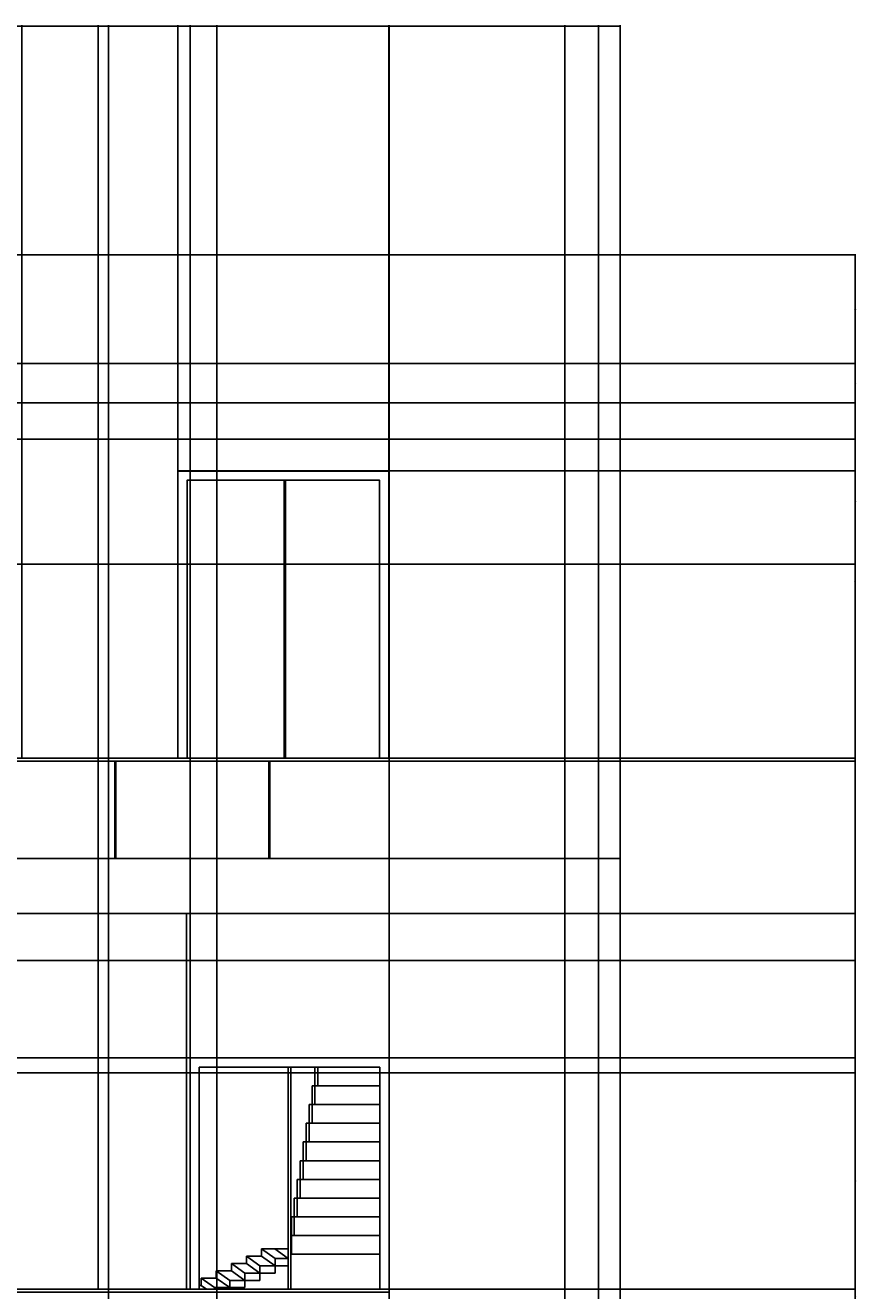
# Model space of a CAD drawing. Units: feet. Extents: x 2193 to 3502, y 890 to 1601.
# Tile 17 of 17: x 3283 to 3502, y 1268 to 1601. Entities that reach past the tile are written whole.
import ezdxf

# ---------------------------------------------------------------- set-up
doc = ezdxf.new("R2010")
doc.units = ezdxf.units.FT
doc.layers.add('A-ANNO-DIMS', color=2, linetype='Continuous', lineweight=18)
doc.layers.add('A-ELEV', color=7, linetype='Continuous', lineweight=25)
doc.styles.get("Standard").update_dxf_attribs({"font": 'arial.ttf'})
doc.dimstyles.get("Standard").update_dxf_attribs({"dimtxt": 0.18, "dimasz": 0.18, "dimexe": 0.18, "dimexo": 0.0625, "dimgap": 0.09, "dimtad": 0, "dimtih": 1, "dimtoh": 1, "dimdec": 0, "dimzin": 0, "dimdsep": 46, "dimlunit": 3, "dimtxsty": 'Standard', "dimcen": 0.09, "dimadec": 0, "dimazin": 0, "dimtfac": 1, "dimtdec": 0, "dimtofl": 0, "dimtmove": 0, "dimatfit": 3, "dimfxl": 1, "dimtolj": 1, "dimtzin": 0, "dimarcsym": 0})

# ---------------------------------------------------------------- blocks, each defined once
blk = doc.blocks.new('STAIR-RAIL-B')
for p, q in [((6.38, 44.29), (6.38, 49.22)), ((5.61, 39.37), (5.61, 44.29)), ((5.61, 44.29), (6.38, 44.29)), ((23.45, 44.29), (6.38, 44.29)), ((6.38, 44.29), (6.38, 39.37)), ((4.83, 34.45), (4.83, 39.37)), ((4.83, 39.37), (5.61, 39.37)), ((23.45, 39.37), (5.61, 39.37)), ((5.61, 39.37), (5.61, 34.45)), ((4.05, 29.53), (4.05, 34.45)), ((4.05, 34.45), (4.83, 34.45)), ((23.45, 34.45), (4.83, 34.45)), ((4.83, 34.45), (4.83, 29.53)), ((3.27, 24.61), (3.27, 29.53)), ((3.27, 29.53), (4.05, 29.53)), ((23.45, 29.53), (4.05, 29.53)), ((4.05, 29.53), (4.05, 24.61)), ((2.49, 19.69), (2.49, 24.61)), ((2.49, 24.61), (3.27, 24.61)), ((23.45, 24.61), (3.27, 24.61)), ((3.27, 24.61), (3.27, 19.69)), ((1.71, 14.77), (1.71, 19.69)), ((1.71, 19.69), (2.49, 19.69)), ((23.45, 19.69), (2.49, 19.69)), ((2.49, 19.69), (2.49, 14.77)), ((0.93, 9.84), (0.93, 14.77)), ((0.93, 14.77), (1.71, 14.77)), ((23.45, 14.77), (1.71, 14.77)), ((1.71, 14.77), (1.71, 9.84)), ((0.15, 4.92), (0.15, 9.84)), ((0.15, 9.84), (0.93, 9.84)), ((23.45, 9.84), (0.93, 9.84)), ((0.93, 9.84), (0.93, 4.92)), ((23.45, 4.92), (0, 4.92)), ((0.15, 4.92), (0.15, 0)), ((23.45, 0), (0, 0))]:
    blk.add_line(p, q)
blk = doc.blocks.new('*D13')
at = {"layer": 'A-ANNO-DIMS', "color": 0, "lineweight": -2, "transparency": 16777216}
for p, q in [((2934.37, 950.89), (2934.37, 1601.47)), ((2934.55, 1601.29), (3186.64, 1601.29)), ((3439.51, 1601.29), (3187.43, 1601.29)), ((3439.69, 1541.11), (3439.69, 1601.47))]:
    blk.add_line(p, q, dxfattribs=at)
at = {"layer": 'A-ANNO-DIMS', "color": 0, "transparency": 16777216}
for points in [[(2934.55, 1601.32), (2934.55, 1601.26), (2934.37, 1601.29)], [(3439.51, 1601.32), (3439.51, 1601.26), (3439.69, 1601.29)]]:
    blk.add_solid(points, dxfattribs=at)
at = {"layer": 'Defpoints', "color": 0, "transparency": 16777216}
for p in [(3439.69, 1601.29), (3439.69, 1541.04), (2934.37, 950.82)]:
    blk.add_point(p, dxfattribs=at)
at = {"layer": 'A-ANNO-DIMS', "color": 0, "transparency": 16777216, "insert": (3187.03, 1601.29), "char_height": 0.18, "attachment_point": 5}
blk.add_mtext('\\A1;505.3', dxfattribs=at)
blk = doc.blocks.new('*D18')
at = {"layer": 'A-ANNO-DIMS', "color": 0, "lineweight": -2, "transparency": 16777216}
for p, q in [((3439.75, 1541.04), (3501.85, 1541.04)), ((3501.67, 1540.86), (3501.67, 1246.12)), ((3501.67, 951), (3501.67, 1245.75)), ((3441.48, 950.82), (3501.85, 950.82))]:
    blk.add_line(p, q, dxfattribs=at)
at = {"layer": 'A-ANNO-DIMS', "color": 0, "transparency": 16777216}
for points in [[(3501.64, 1540.86), (3501.7, 1540.86), (3501.67, 1541.04)], [(3501.64, 951), (3501.7, 951), (3501.67, 950.82)]]:
    blk.add_solid(points, dxfattribs=at)
at = {"layer": 'Defpoints', "color": 0, "transparency": 16777216}
for p in [(3439.69, 1541.04), (3501.67, 1541.04), (3441.42, 950.82)]:
    blk.add_point(p, dxfattribs=at)
at = {"layer": 'A-ANNO-DIMS', "color": 0, "transparency": 16777216, "insert": (3501.67, 1245.93), "char_height": 0.18, "attachment_point": 5}
blk.add_mtext('\\A1;590.2', dxfattribs=at)
blk = doc.blocks.new('*D31')
at = {"layer": 'A-ANNO-DIMS', "color": 0, "lineweight": -2, "transparency": 16777216}
for p, q in [((2760.54, 1541.04), (3501.85, 1541.04)), ((3501.67, 1540.86), (3501.67, 1246.12)), ((3501.67, 951), (3501.67, 1245.75)), ((2762.27, 950.82), (3501.85, 950.82))]:
    blk.add_line(p, q, dxfattribs=at)
at = {"layer": 'A-ANNO-DIMS', "color": 0, "transparency": 16777216}
for points in [[(3501.64, 1540.86), (3501.7, 1540.86), (3501.67, 1541.04)], [(3501.64, 951), (3501.7, 951), (3501.67, 950.82)]]:
    blk.add_solid(points, dxfattribs=at)
at = {"layer": 'Defpoints', "color": 0, "transparency": 16777216}
for p in [(2760.47, 1541.04), (3501.67, 1541.04), (2762.2, 950.82)]:
    blk.add_point(p, dxfattribs=at)
at = {"layer": 'A-ANNO-DIMS', "color": 0, "transparency": 16777216, "insert": (3501.67, 1245.93), "char_height": 0.18, "attachment_point": 5}
blk.add_mtext('\\A1;590.2', dxfattribs=at)
blk = doc.blocks.new('*D40')
at = {"layer": 'A-ANNO-DIMS', "color": 0, "lineweight": -2, "transparency": 16777216}
for p, q in [((3378.91, 1502.08), (3501.85, 1502.08)), ((3501.67, 1501.9), (3501.67, 1455.09)), ((3501.67, 1407.92), (3501.67, 1454.73)), ((3378.85, 1407.74), (3501.85, 1407.74))]:
    blk.add_line(p, q, dxfattribs=at)
at = {"layer": 'A-ANNO-DIMS', "color": 0, "transparency": 16777216}
for points in [[(3501.64, 1501.9), (3501.7, 1501.9), (3501.67, 1502.08)], [(3501.64, 1407.92), (3501.7, 1407.92), (3501.67, 1407.74)]]:
    blk.add_solid(points, dxfattribs=at)
at = {"layer": 'Defpoints', "color": 0, "transparency": 16777216}
for p in [(3378.85, 1502.08), (3501.67, 1502.08), (3378.79, 1407.74)]:
    blk.add_point(p, dxfattribs=at)
at = {"layer": 'A-ANNO-DIMS', "color": 0, "transparency": 16777216, "insert": (3501.67, 1454.91), "char_height": 0.18, "attachment_point": 5}
blk.add_mtext('\\A1;94.34', dxfattribs=at)
blk = doc.blocks.new('*D41')
at = {"layer": 'A-ANNO-DIMS', "color": 0, "lineweight": -2, "transparency": 16777216}
for p, q in [((3439.75, 1512.4), (3501.85, 1512.4)), ((3501.67, 1512.22), (3501.67, 1507.42)), ((3501.67, 1502.26), (3501.67, 1507.05)), ((3378.91, 1502.08), (3501.85, 1502.08))]:
    blk.add_line(p, q, dxfattribs=at)
at = {"layer": 'A-ANNO-DIMS', "color": 0, "transparency": 16777216}
for points in [[(3501.64, 1512.22), (3501.7, 1512.22), (3501.67, 1512.4)], [(3501.64, 1502.26), (3501.7, 1502.26), (3501.67, 1502.08)]]:
    blk.add_solid(points, dxfattribs=at)
at = {"layer": 'Defpoints', "color": 0, "transparency": 16777216}
for p in [(3439.69, 1512.4), (3501.67, 1512.4), (3378.85, 1502.08)]:
    blk.add_point(p, dxfattribs=at)
at = {"layer": 'A-ANNO-DIMS', "color": 0, "transparency": 16777216, "insert": (3501.67, 1507.24), "char_height": 0.18, "attachment_point": 5}
blk.add_mtext('\\A1;10.32', dxfattribs=at)
blk = doc.blocks.new('*D42')
at = {"layer": 'A-ANNO-DIMS', "color": 0, "lineweight": -2, "transparency": 16777216}
for p, q in [((3439.75, 1541.04), (3501.85, 1541.04)), ((3501.67, 1540.86), (3501.67, 1526.9)), ((3501.67, 1512.58), (3501.67, 1526.54)), ((3439.75, 1512.4), (3501.85, 1512.4))]:
    blk.add_line(p, q, dxfattribs=at)
at = {"layer": 'A-ANNO-DIMS', "color": 0, "transparency": 16777216}
for points in [[(3501.64, 1540.86), (3501.7, 1540.86), (3501.67, 1541.04)], [(3501.64, 1512.58), (3501.7, 1512.58), (3501.67, 1512.4)]]:
    blk.add_solid(points, dxfattribs=at)
at = {"layer": 'Defpoints', "color": 0, "transparency": 16777216}
for p in [(3439.69, 1541.04), (3501.67, 1541.04), (3439.69, 1512.4)]:
    blk.add_point(p, dxfattribs=at)
at = {"layer": 'A-ANNO-DIMS', "color": 0, "transparency": 16777216, "insert": (3501.67, 1526.72), "char_height": 0.18, "attachment_point": 5}
blk.add_mtext('\\A1;28.65', dxfattribs=at)
blk = doc.blocks.new('*D44')
at = {"layer": 'A-ANNO-DIMS', "color": 0, "lineweight": -2, "transparency": 16777216}
for p, q in [((3282.08, 1502.14), (3282.08, 1601.47)), ((3282.26, 1601.29), (3330.07, 1601.29)), ((3378.67, 1601.29), (3330.86, 1601.29)), ((3378.85, 1502.14), (3378.85, 1601.47))]:
    blk.add_line(p, q, dxfattribs=at)
at = {"layer": 'A-ANNO-DIMS', "color": 0, "transparency": 16777216}
for points in [[(3282.26, 1601.32), (3282.26, 1601.26), (3282.08, 1601.29)], [(3378.67, 1601.32), (3378.67, 1601.26), (3378.85, 1601.29)]]:
    blk.add_solid(points, dxfattribs=at)
at = {"layer": 'Defpoints', "color": 0, "transparency": 16777216}
for p in [(3378.85, 1601.29), (3282.08, 1502.08), (3378.85, 1502.08)]:
    blk.add_point(p, dxfattribs=at)
at = {"layer": 'A-ANNO-DIMS', "color": 0, "transparency": 16777216, "insert": (3330.47, 1601.29), "char_height": 0.18, "attachment_point": 5}
blk.add_mtext('\\A1;96.77', dxfattribs=at)
blk = doc.blocks.new('*D45')
at = {"layer": 'A-ANNO-DIMS', "color": 0, "lineweight": -2, "transparency": 16777216}
for p, q in [((3378.85, 1502.14), (3378.85, 1601.47)), ((3379.03, 1601.29), (3408.88, 1601.29)), ((3439.51, 1601.29), (3409.66, 1601.29)), ((3439.69, 1541.11), (3439.69, 1601.47))]:
    blk.add_line(p, q, dxfattribs=at)
at = {"layer": 'A-ANNO-DIMS', "color": 0, "transparency": 16777216}
for points in [[(3379.03, 1601.32), (3379.03, 1601.26), (3378.85, 1601.29)], [(3439.51, 1601.32), (3439.51, 1601.26), (3439.69, 1601.29)]]:
    blk.add_solid(points, dxfattribs=at)
at = {"layer": 'Defpoints', "color": 0, "transparency": 16777216}
for p in [(3439.69, 1601.29), (3439.69, 1541.04), (3378.85, 1502.08)]:
    blk.add_point(p, dxfattribs=at)
at = {"layer": 'A-ANNO-DIMS', "color": 0, "transparency": 16777216, "insert": (3409.27, 1601.29), "char_height": 0.18, "attachment_point": 5}
blk.add_mtext('\\A1;60.84', dxfattribs=at)
blk = doc.blocks.new('*D46')
at = {"layer": 'A-ANNO-DIMS', "color": 0, "lineweight": -2, "transparency": 16777216}
for p, q in [((3323.18, 1484.18), (3323.18, 1601.47)), ((3323.36, 1601.29), (3350.66, 1601.29)), ((3378.61, 1601.29), (3351.31, 1601.29)), ((3378.79, 1484.18), (3378.79, 1601.47))]:
    blk.add_line(p, q, dxfattribs=at)
at = {"layer": 'A-ANNO-DIMS', "color": 0, "transparency": 16777216}
for points in [[(3323.36, 1601.32), (3323.36, 1601.26), (3323.18, 1601.29)], [(3378.61, 1601.32), (3378.61, 1601.26), (3378.79, 1601.29)]]:
    blk.add_solid(points, dxfattribs=at)
at = {"layer": 'Defpoints', "color": 0, "transparency": 16777216}
for p in [(3378.79, 1601.29), (3323.18, 1484.12), (3378.79, 1484.12)]:
    blk.add_point(p, dxfattribs=at)
at = {"layer": 'A-ANNO-DIMS', "color": 0, "transparency": 16777216, "insert": (3350.99, 1601.29), "char_height": 0.18, "attachment_point": 5}
blk.add_mtext('\\A1;55.6', dxfattribs=at)
blk = doc.blocks.new('*D47')
at = {"layer": 'A-ANNO-DIMS', "color": 0, "lineweight": -2, "transparency": 16777216}
for p, q in [((3323.25, 1484.12), (3501.85, 1484.12)), ((3501.67, 1483.94), (3501.67, 1446.48)), ((3501.67, 1408.66), (3501.67, 1446.12)), ((3323.25, 1408.48), (3501.85, 1408.48))]:
    blk.add_line(p, q, dxfattribs=at)
at = {"layer": 'A-ANNO-DIMS', "color": 0, "transparency": 16777216}
for points in [[(3501.64, 1483.94), (3501.7, 1483.94), (3501.67, 1484.12)], [(3501.64, 1408.66), (3501.7, 1408.66), (3501.67, 1408.48)]]:
    blk.add_solid(points, dxfattribs=at)
at = {"layer": 'Defpoints', "color": 0, "transparency": 16777216}
for p in [(3323.18, 1484.12), (3501.67, 1484.12), (3323.18, 1408.48)]:
    blk.add_point(p, dxfattribs=at)
at = {"layer": 'A-ANNO-DIMS', "color": 0, "transparency": 16777216, "insert": (3501.67, 1446.3), "char_height": 0.18, "attachment_point": 5}
blk.add_mtext('\\A1;75.63', dxfattribs=at)
blk = doc.blocks.new('*D51')
at = {"layer": 'A-ANNO-DIMS', "color": 0, "lineweight": -2, "transparency": 16777216}
for p, q in [((2965.78, 1492.51), (3501.85, 1492.51)), ((3501.67, 1492.33), (3501.67, 1476.24)), ((3501.67, 1459.78), (3501.67, 1475.88)), ((3001.96, 1459.6), (3501.85, 1459.6))]:
    blk.add_line(p, q, dxfattribs=at)
at = {"layer": 'A-ANNO-DIMS', "color": 0, "transparency": 16777216}
for points in [[(3501.64, 1492.33), (3501.7, 1492.33), (3501.67, 1492.51)], [(3501.64, 1459.78), (3501.7, 1459.78), (3501.67, 1459.6)]]:
    blk.add_solid(points, dxfattribs=at)
at = {"layer": 'Defpoints', "color": 0, "transparency": 16777216}
for p in [(2965.72, 1492.51), (3501.67, 1492.51), (3001.89, 1459.6)]:
    blk.add_point(p, dxfattribs=at)
at = {"layer": 'A-ANNO-DIMS', "color": 0, "transparency": 16777216, "insert": (3501.67, 1476.06), "char_height": 0.18, "attachment_point": 5}
blk.add_mtext('\\A1;32.91', dxfattribs=at)
blk = doc.blocks.new('*D60')
at = {"layer": 'A-ANNO-DIMS', "color": 0, "lineweight": -2, "transparency": 16777216}
for p, q in [((3070.17, 1329.58), (3501.85, 1329.58)), ((3501.67, 1329.4), (3501.67, 1299.3)), ((3501.67, 1268.84), (3501.67, 1298.94)), ((3070.17, 1268.66), (3501.85, 1268.66))]:
    blk.add_line(p, q, dxfattribs=at)
at = {"layer": 'A-ANNO-DIMS', "color": 0, "transparency": 16777216}
for points in [[(3501.64, 1329.4), (3501.7, 1329.4), (3501.67, 1329.58)], [(3501.64, 1268.84), (3501.7, 1268.84), (3501.67, 1268.66)]]:
    blk.add_solid(points, dxfattribs=at)
at = {"layer": 'Defpoints', "color": 0, "transparency": 16777216}
for p in [(3070.11, 1329.58), (3501.67, 1329.58), (3070.11, 1268.66)]:
    blk.add_point(p, dxfattribs=at)
at = {"layer": 'A-ANNO-DIMS', "color": 0, "transparency": 16777216, "insert": (3501.67, 1299.12), "char_height": 0.18, "attachment_point": 5}
blk.add_mtext('\\A1;60.92', dxfattribs=at)
blk = doc.blocks.new('*D68')
at = {"layer": 'A-ANNO-DIMS', "color": 0, "lineweight": -2, "transparency": 16777216}
for p, q in [((3378.85, 1367.64), (3378.85, 1601.47)), ((3379.03, 1601.29), (3401.62, 1601.29)), ((3425.01, 1601.29), (3402.42, 1601.29)), ((3425.19, 1367.64), (3425.19, 1601.47))]:
    blk.add_line(p, q, dxfattribs=at)
at = {"layer": 'A-ANNO-DIMS', "color": 0, "transparency": 16777216}
for points in [[(3379.03, 1601.32), (3379.03, 1601.26), (3378.85, 1601.29)], [(3425.01, 1601.32), (3425.01, 1601.26), (3425.19, 1601.29)]]:
    blk.add_solid(points, dxfattribs=at)
at = {"layer": 'Defpoints', "color": 0, "transparency": 16777216}
for p in [(3425.19, 1601.29), (3378.85, 1367.57), (3425.19, 1367.57)]:
    blk.add_point(p, dxfattribs=at)
at = {"layer": 'A-ANNO-DIMS', "color": 0, "transparency": 16777216, "insert": (3402.02, 1601.29), "char_height": 0.18, "attachment_point": 5}
blk.add_mtext('\\A1;46.34', dxfattribs=at)
blk = doc.blocks.new('*D69')
at = {"layer": 'A-ANNO-DIMS', "color": 0, "lineweight": -2, "transparency": 16777216}
for p, q in [((3425.25, 1367.57), (3501.85, 1367.57)), ((3501.67, 1367.39), (3501.67, 1267.09)), ((3501.67, 1166.41), (3501.67, 1266.72)), ((3425.25, 1166.23), (3501.85, 1166.23))]:
    blk.add_line(p, q, dxfattribs=at)
at = {"layer": 'A-ANNO-DIMS', "color": 0, "transparency": 16777216}
for points in [[(3501.64, 1367.39), (3501.7, 1367.39), (3501.67, 1367.57)], [(3501.64, 1166.41), (3501.7, 1166.41), (3501.67, 1166.23)]]:
    blk.add_solid(points, dxfattribs=at)
at = {"layer": 'Defpoints', "color": 0, "transparency": 16777216}
for p in [(3425.19, 1367.57), (3501.67, 1367.57), (3425.19, 1166.23)]:
    blk.add_point(p, dxfattribs=at)
at = {"layer": 'A-ANNO-DIMS', "color": 0, "transparency": 16777216, "insert": (3501.67, 1266.9), "char_height": 0.18, "attachment_point": 5}
blk.add_mtext('\\A1;201.34', dxfattribs=at)
blk = doc.blocks.new('*D71')
at = {"layer": 'A-ANNO-DIMS', "color": 0, "lineweight": -2, "transparency": 16777216}
for p, q in [((3132, 1355.28), (3132, 1601.47)), ((3132.18, 1601.29), (3216.71, 1601.29)), ((3302.02, 1601.29), (3217.48, 1601.29)), ((3302.2, 1355.28), (3302.2, 1601.47))]:
    blk.add_line(p, q, dxfattribs=at)
at = {"layer": 'A-ANNO-DIMS', "color": 0, "transparency": 16777216}
for points in [[(3132.18, 1601.32), (3132.18, 1601.26), (3132, 1601.29)], [(3302.02, 1601.32), (3302.02, 1601.26), (3302.2, 1601.29)]]:
    blk.add_solid(points, dxfattribs=at)
at = {"layer": 'Defpoints', "color": 0, "transparency": 16777216}
for p in [(3302.2, 1601.29), (3132, 1355.22), (3302.2, 1355.22)]:
    blk.add_point(p, dxfattribs=at)
at = {"layer": 'A-ANNO-DIMS', "color": 0, "transparency": 16777216, "insert": (3217.1, 1601.29), "char_height": 0.18, "attachment_point": 5}
blk.add_mtext('\\A1;170.2', dxfattribs=at)
blk = doc.blocks.new('*D72')
at = {"layer": 'A-ANNO-DIMS', "color": 0, "lineweight": -2, "transparency": 16777216}
for p, q in [((3302.26, 1355.22), (3501.85, 1355.22)), ((3501.67, 1355.04), (3501.67, 1312.12)), ((3501.67, 1268.84), (3501.67, 1311.76)), ((3302.26, 1268.66), (3501.85, 1268.66))]:
    blk.add_line(p, q, dxfattribs=at)
at = {"layer": 'A-ANNO-DIMS', "color": 0, "transparency": 16777216}
for points in [[(3501.64, 1355.04), (3501.7, 1355.04), (3501.67, 1355.22)], [(3501.64, 1268.84), (3501.7, 1268.84), (3501.67, 1268.66)]]:
    blk.add_solid(points, dxfattribs=at)
at = {"layer": 'Defpoints', "color": 0, "transparency": 16777216}
for p in [(3302.2, 1355.22), (3501.67, 1355.22), (3302.2, 1268.66)]:
    blk.add_point(p, dxfattribs=at)
at = {"layer": 'A-ANNO-DIMS', "color": 0, "transparency": 16777216, "insert": (3501.67, 1311.94), "char_height": 0.18, "attachment_point": 5}
blk.add_mtext('\\A1;86.56', dxfattribs=at)
blk = doc.blocks.new('*D75')
at = {"layer": 'A-ANNO-DIMS', "color": 0, "lineweight": -2, "transparency": 16777216}
for p, q in [((3259.05, 1325.67), (3501.85, 1325.67)), ((3501.67, 1325.49), (3501.67, 1297.35)), ((3501.67, 1268.84), (3501.67, 1296.98)), ((3259.05, 1268.66), (3501.85, 1268.66))]:
    blk.add_line(p, q, dxfattribs=at)
at = {"layer": 'A-ANNO-DIMS', "color": 0, "transparency": 16777216}
for points in [[(3501.64, 1325.49), (3501.7, 1325.49), (3501.67, 1325.67)], [(3501.64, 1268.84), (3501.7, 1268.84), (3501.67, 1268.66)]]:
    blk.add_solid(points, dxfattribs=at)
at = {"layer": 'Defpoints', "color": 0, "transparency": 16777216}
for p in [(3258.98, 1325.67), (3501.67, 1325.67), (3258.98, 1268.66)]:
    blk.add_point(p, dxfattribs=at)
at = {"layer": 'A-ANNO-DIMS', "color": 0, "transparency": 16777216, "insert": (3501.67, 1297.16), "char_height": 0.18, "attachment_point": 5}
blk.add_mtext('\\A1;57.01', dxfattribs=at)
blk = doc.blocks.new('*D77')
at = {"layer": 'A-ANNO-DIMS', "color": 0, "lineweight": -2, "transparency": 16777216}
for p, q in [((3326.4, 1329.64), (3326.4, 1601.47)), ((3326.58, 1601.29), (3352.23, 1601.29)), ((3378.67, 1601.29), (3353.02, 1601.29)), ((3378.85, 1329.64), (3378.85, 1601.47))]:
    blk.add_line(p, q, dxfattribs=at)
at = {"layer": 'A-ANNO-DIMS', "color": 0, "transparency": 16777216}
for points in [[(3326.58, 1601.32), (3326.58, 1601.26), (3326.4, 1601.29)], [(3378.67, 1601.32), (3378.67, 1601.26), (3378.85, 1601.29)]]:
    blk.add_solid(points, dxfattribs=at)
at = {"layer": 'Defpoints', "color": 0, "transparency": 16777216}
for p in [(3378.85, 1601.29), (3326.4, 1329.58), (3378.85, 1329.58)]:
    blk.add_point(p, dxfattribs=at)
at = {"layer": 'A-ANNO-DIMS', "color": 0, "transparency": 16777216, "insert": (3352.62, 1601.29), "char_height": 0.18, "attachment_point": 5}
blk.add_mtext('\\A1;52.45', dxfattribs=at)
blk = doc.blocks.new('*D78')
at = {"layer": 'A-ANNO-DIMS', "color": 0, "lineweight": -2, "transparency": 16777216}
for p, q in [((3326.46, 1329.58), (3501.85, 1329.58)), ((3501.67, 1329.4), (3501.67, 1299.3)), ((3501.67, 1268.84), (3501.67, 1298.94)), ((3326.46, 1268.66), (3501.85, 1268.66))]:
    blk.add_line(p, q, dxfattribs=at)
at = {"layer": 'A-ANNO-DIMS', "color": 0, "transparency": 16777216}
for points in [[(3501.64, 1329.4), (3501.7, 1329.4), (3501.67, 1329.58)], [(3501.64, 1268.84), (3501.7, 1268.84), (3501.67, 1268.66)]]:
    blk.add_solid(points, dxfattribs=at)
at = {"layer": 'Defpoints', "color": 0, "transparency": 16777216}
for p in [(3326.4, 1329.58), (3501.67, 1329.58), (3326.4, 1268.66)]:
    blk.add_point(p, dxfattribs=at)
at = {"layer": 'A-ANNO-DIMS', "color": 0, "transparency": 16777216, "insert": (3501.67, 1299.12), "char_height": 0.18, "attachment_point": 5}
blk.add_mtext('\\A1;60.92', dxfattribs=at)
blk = doc.blocks.new('*D97')
at = {"layer": 'A-ANNO-DIMS', "color": 0, "lineweight": -2, "transparency": 16777216}
for p, q in [((3111.13, 1032.26), (3111.13, 1601.47)), ((3111.31, 1601.29), (3207.6, 1601.29)), ((3304.79, 1601.29), (3208.51, 1601.29)), ((3304.97, 1032.26), (3304.97, 1601.47))]:
    blk.add_line(p, q, dxfattribs=at)
at = {"layer": 'A-ANNO-DIMS', "color": 0, "transparency": 16777216}
for points in [[(3111.31, 1601.32), (3111.31, 1601.26), (3111.13, 1601.29)], [(3304.79, 1601.32), (3304.79, 1601.26), (3304.97, 1601.29)]]:
    blk.add_solid(points, dxfattribs=at)
at = {"layer": 'Defpoints', "color": 0, "transparency": 16777216}
for p in [(3304.97, 1601.29), (3111.13, 1032.19), (3304.97, 1032.19)]:
    blk.add_point(p, dxfattribs=at)
at = {"layer": 'A-ANNO-DIMS', "color": 0, "transparency": 16777216, "insert": (3208.05, 1601.29), "char_height": 0.18, "attachment_point": 5}
blk.add_mtext('\\A1;193.84', dxfattribs=at)
blk = doc.blocks.new('*D123')
at = {"layer": 'A-ANNO-DIMS', "color": 0, "lineweight": -2, "transparency": 16777216}
for p, q in [((3433.98, 1073.09), (3433.98, 1601.47)), ((3434.16, 1601.29), (3436.44, 1601.29)), ((3439.51, 1601.29), (3437.23, 1601.29)), ((3439.69, 1073.09), (3439.69, 1601.47))]:
    blk.add_line(p, q, dxfattribs=at)
at = {"layer": 'A-ANNO-DIMS', "color": 0, "transparency": 16777216}
for points in [[(3434.16, 1601.32), (3434.16, 1601.26), (3433.98, 1601.29)], [(3439.51, 1601.32), (3439.51, 1601.26), (3439.69, 1601.29)]]:
    blk.add_solid(points, dxfattribs=at)
at = {"layer": 'Defpoints', "color": 0, "transparency": 16777216}
for p in [(3439.69, 1601.29), (3433.98, 1073.03), (3439.69, 1073.03)]:
    blk.add_point(p, dxfattribs=at)
at = {"layer": 'A-ANNO-DIMS', "color": 0, "transparency": 16777216, "insert": (3436.84, 1601.29), "char_height": 0.18, "attachment_point": 5}
blk.add_mtext('\\A1;5.707', dxfattribs=at)
blk = doc.blocks.new('*D125')
at = {"layer": 'A-ANNO-DIMS', "color": 0, "lineweight": -2, "transparency": 16777216}
for p, q in [((3304.97, 1073.09), (3304.97, 1601.47)), ((3305.15, 1601.29), (3318.84, 1601.29)), ((3333.32, 1601.29), (3319.63, 1601.29)), ((3333.5, 1073.09), (3333.5, 1601.47))]:
    blk.add_line(p, q, dxfattribs=at)
at = {"layer": 'A-ANNO-DIMS', "color": 0, "transparency": 16777216}
for points in [[(3305.15, 1601.32), (3305.15, 1601.26), (3304.97, 1601.29)], [(3333.32, 1601.32), (3333.32, 1601.26), (3333.5, 1601.29)]]:
    blk.add_solid(points, dxfattribs=at)
at = {"layer": 'Defpoints', "color": 0, "transparency": 16777216}
for p in [(3333.5, 1601.29), (3304.97, 1073.03), (3333.5, 1073.03)]:
    blk.add_point(p, dxfattribs=at)
at = {"layer": 'A-ANNO-DIMS', "color": 0, "transparency": 16777216, "insert": (3319.24, 1601.29), "char_height": 0.18, "attachment_point": 5}
blk.add_mtext('\\A1;28.53', dxfattribs=at)

msp = doc.modelspace()

# ---------------------------------------------------------------- linework, layer by layer
at = {"layer": 'A-ELEV'}
for p, q in [((3439.6901, 1541.0441), (3378.849, 1541.0441)), ((3378.849, 1512.3957), (3378.849, 1541.0441)), ((3439.6901, 1382.0763), (3439.6901, 1541.0441)), ((3439.6901, 1502.0763), (3265.3903, 1502.0763)), ((3439.6901, 956.8829), (3439.6901, 1494.0584)), ((3215.7583, 1367.5739), (3325.5011, 1367.5739)), ((3131.9988, 1355.2199), (3302.1981, 1355.2199)), ((3360.1133, 1327.1314), (3360.1133, 1322.2098)), ((3341.2875, 1275.4405), (3341.2875, 1277.358)), ((3341.2875, 1277.358), (3345.27, 1277.358)), ((3344.8379, 1274.8393), (3341.2875, 1277.358)), ((3348.8205, 1276.7569), (3345.27, 1279.2756)), ((3345.27, 1279.2756), (3348.7495, 1279.2756)), ((3345.27, 1277.358), (3345.27, 1279.2756)), ((3345.27, 1277.358), (3348.8205, 1274.8393)), ((3348.7495, 1279.2756), (3352.2999, 1276.7569)), ((3348.7495, 1279.2756), (3352.2999, 1279.2756)), ((3348.8205, 1274.8393), (3348.8205, 1276.7569)), ((3348.8205, 1276.7569), (3352.2999, 1276.7569)), ((3333.3223, 1271.6053), (3333.3223, 1273.5229)), ((3333.3223, 1273.5229), (3337.3049, 1273.5229)), ((3333.3223, 1273.5229), (3336.8727, 1271.0041)), ((3337.3049, 1273.5229), (3337.3049, 1275.4405)), ((3337.3049, 1275.4405), (3341.2875, 1275.4405)), ((3337.3049, 1275.4405), (3340.8553, 1272.9217)), ((3337.3049, 1273.5229), (3340.8553, 1271.0041)), ((3340.8553, 1271.0041), (3340.8553, 1272.9217)), ((3340.8553, 1272.9217), (3344.8379, 1272.9217)), ((3341.2875, 1275.4405), (3344.8379, 1272.9217)), ((3344.8379, 1272.9217), (3344.8379, 1274.8393)), ((3344.8379, 1274.8393), (3348.8205, 1274.8393)), ((3344.8379, 1271.0041), (3344.8379, 1272.9217)), ((3344.8379, 1272.9217), (3348.8205, 1272.9217)), ((3348.8205, 1274.8393), (3352.2999, 1274.8393)), ((3348.8205, 1272.9217), (3348.8205, 1274.8393)), ((3328.846, 1269.6877), (3329.3397, 1269.6877)), ((3329.3397, 1269.6877), (3329.3397, 1271.6053)), ((3329.3397, 1271.6053), (3333.3223, 1271.6053)), ((3329.3397, 1271.6053), (3332.8902, 1269.0866)), ((3329.3397, 1269.6877), (3330.7886, 1268.6599)), ((3333.3223, 1271.6053), (3336.8727, 1269.0866)), ((3336.8727, 1269.0866), (3336.8727, 1271.0041)), ((3336.8727, 1271.0041), (3340.8553, 1271.0041)), ((3340.8553, 1269.0866), (3340.8553, 1271.0041)), ((3340.8553, 1271.0041), (3344.8379, 1271.0041)), ((3332.8902, 1268.6599), (3332.8902, 1269.0866)), ((3332.8902, 1269.0866), (3336.8727, 1269.0866)), ((3336.8727, 1268.6599), (3336.8727, 1269.0866)), ((3336.8727, 1269.0866), (3340.8553, 1269.0866))]:
    msp.add_line(p, q, dxfattribs=at)
for points in [[(3282.0816, 1502.0763), (3265.3903, 1502.0763), (3265.3903, 1512.3957), (3439.6901, 1512.3957), (3439.6901, 1502.0763)], [(3378.849, 1502.0763), (3378.7894, 1502.0763)], [(3378.849, 1382.0763), (3378.849, 1502.0763)], [(3325.63, 1408.4814), (3325.63, 1481.67), (3376.3443, 1481.67), (3376.3443, 1408.4814)], [(3439.6901, 1415.3157), (3439.6901, 1089.3627), (3378.849, 1089.3627), (3378.849, 1367.5739)], [(3215.7583, 1408.4814), (3378.7894, 1408.4814)], [(3378.7894, 1407.7384), (3215.7583, 1407.7384)], [(3306.8213, 1407.7384), (3306.8213, 1382.0763), (3306.5716, 1382.0763), (3306.5716, 1407.7384)], [(3347.39, 1407.7384), (3347.39, 1382.0763), (3347.1403, 1382.0763), (3347.1403, 1407.7384)], [(3425.1877, 1367.5739), (2954.2649, 1367.5739), (2954.2649, 1382.0763), (3439.6901, 1382.0763), (3439.6901, 1367.5739)], [(3302.1981, 1367.5739), (3325.5011, 1367.5739), (3325.5011, 1268.6599), (3302.1981, 1268.6599), (3302.1981, 1355.2199)], [(3425.1877, 1166.2327), (3425.1877, 1367.5739)], [(3328.846, 1268.6599), (3328.846, 1327.1314), (3376.4039, 1327.1314), (3376.4039, 1268.6599)], [(3378.849, 1267.9169), (3147.5022, 1267.9169), (3147.5022, 1268.6599), (3378.849, 1268.6599)]]:
    msp.add_lwpolyline(points, dxfattribs=at)
for points in [[(3378.7894, 1408.4814), (3282.0816, 1408.4814), (3282.0816, 1502.0763), (3378.7894, 1502.0763)], [(3378.7894, 1408.4814), (3323.1849, 1408.4814), (3323.1849, 1484.1152), (3378.7894, 1484.1152)], [(3351.1858, 1481.67), (3351.5831, 1481.67), (3351.5831, 1408.4814), (3351.1858, 1408.4814)], [(3378.849, 1268.6599), (3326.4009, 1268.6599), (3326.4009, 1329.5765), (3378.849, 1329.5765)], [(3352.2999, 1327.1314), (3352.95, 1327.1314), (3352.95, 1268.6599), (3352.2999, 1268.6599)]]:
    msp.add_lwpolyline(points, close=True, dxfattribs=at)

# ---------------------------------------------------------------- block references
msp.add_blockref('STAIR-RAIL-B', (3352.95, 1277.9151), dxfattribs=at)

# ---------------------------------------------------------------- dimensions: what is measured, and where the dimension line sits
at = {"layer": 'A-ANNO-DIMS'}
for base, p1, p2, override, picture, middle in [((3439.6901, 1601.2941), (2934.3742, 950.8228), (3439.6901, 1541.0441), {"dimdec": 1, "dimlfac": 1, "dimrnd": 0, "dimzin": 0, "dimdsep": 46, "dimlunit": 2}, '*D13', (3187.0321, 1601.2941)), ((3304.9731, 1601.2941), (3111.1302, 1032.1935), (3304.9731, 1032.1935), {"dimdec": 2, "dimlfac": 1, "dimrnd": 0, "dimzin": 0, "dimdsep": 46, "dimlunit": 2}, '*D97', (3208.0516, 1601.2941)), ((3302.1981, 1601.2941), (3131.9988, 1355.2199), (3302.1981, 1355.2199), {"dimdec": 1, "dimlfac": 1, "dimrnd": 0, "dimzin": 0, "dimdsep": 46, "dimlunit": 2}, '*D71', (3217.0985, 1601.2941)), ((3378.849, 1601.2941), (3282.0816, 1502.0763), (3378.849, 1502.0763), {"dimdec": 2, "dimlfac": 1, "dimrnd": 0, "dimzin": 0, "dimdsep": 46, "dimlunit": 2}, '*D44', (3330.4653, 1601.2941)), ((3333.5009, 1601.2941), (3304.9731, 1073.031), (3333.5009, 1073.031), {"dimdec": 2, "dimlfac": 1, "dimrnd": 0, "dimzin": 0, "dimdsep": 46, "dimlunit": 2}, '*D125', (3319.237, 1601.2941)), ((3378.7894, 1601.2941), (3323.1849, 1484.1152), (3378.7894, 1484.1152), {"dimdec": 1, "dimlfac": 1, "dimrnd": 0, "dimzin": 0, "dimdsep": 46, "dimlunit": 2}, '*D46', (3350.9871, 1601.2941)), ((3378.849, 1601.2941), (3326.4009, 1329.5765), (3378.849, 1329.5765), {"dimdec": 2, "dimlfac": 1, "dimrnd": 0, "dimzin": 0, "dimdsep": 46, "dimlunit": 2}, '*D77', (3352.6249, 1601.2941)), ((3439.6901, 1601.2941), (3378.849, 1502.0763), (3439.6901, 1541.0441), {"dimdec": 2, "dimlfac": 1, "dimrnd": 0, "dimzin": 0, "dimdsep": 46, "dimlunit": 2}, '*D45', (3409.2695, 1601.2941)), ((3425.1877, 1601.2941), (3378.849, 1367.5739), (3425.1877, 1367.5739), {"dimdec": 2, "dimlfac": 1, "dimrnd": 0, "dimzin": 0, "dimdsep": 46, "dimlunit": 2}, '*D68', (3402.0184, 1601.2941)), ((3439.6901, 1601.2941), (3433.9829, 1073.031), (3439.6901, 1073.031), {"dimdec": 3, "dimlfac": 1, "dimrnd": 0, "dimzin": 0, "dimdsep": 46, "dimlunit": 2}, '*D123', (3436.8365, 1601.2941))]:
    dim = msp.add_linear_dim(base=base, p1=p1, p2=p2, dimstyle='Standard', override=override, dxfattribs=at)
    dim.commit()
    dim.dimension.update_dxf_attribs({"geometry": picture, "text_midpoint": middle})
for base, p1, p2, override, picture, middle in [((3501.6716, 1541.0441), (2762.2048, 950.8228), (2760.4733, 1541.0441), {"dimdec": 1, "dimlfac": 1, "dimrnd": 0, "dimzin": 0, "dimdsep": 46, "dimlunit": 2}, '*D31', (3501.6716, 1245.9334)), ((3501.6716, 1541.0441), (3441.4216, 950.8228), (3439.6901, 1541.0441), {"dimdec": 1, "dimlfac": 1, "dimrnd": 0, "dimzin": 0, "dimdsep": 46, "dimlunit": 2}, '*D18', (3501.6716, 1245.9334)), ((3501.6716, 1541.0441), (3439.6901, 1512.3957), (3439.6901, 1541.0441), {"dimdec": 2, "dimlfac": 1, "dimrnd": 0, "dimzin": 0, "dimdsep": 46, "dimlunit": 2}, '*D42', (3501.6716, 1526.7199)), ((3501.6716, 1512.3957), (3378.849, 1502.0763), (3439.6901, 1512.3957), {"dimdec": 2, "dimlfac": 1, "dimrnd": 0, "dimzin": 0, "dimdsep": 46, "dimlunit": 2}, '*D41', (3501.6716, 1507.236)), ((3501.6716, 1502.0763), (3378.7894, 1407.7384), (3378.849, 1502.0763), {"dimdec": 2, "dimlfac": 1, "dimrnd": 0, "dimzin": 0, "dimdsep": 46, "dimlunit": 2}, '*D40', (3501.6716, 1454.9074)), ((3501.6716, 1492.5146), (3001.8944, 1459.6035), (2965.7197, 1492.5146), {"dimdec": 2, "dimlfac": 1, "dimrnd": 0, "dimzin": 0, "dimdsep": 46, "dimlunit": 2}, '*D51', (3501.6716, 1476.0591)), ((3501.6716, 1484.1152), (3323.1849, 1408.4814), (3323.1849, 1484.1152), {"dimdec": 2, "dimlfac": 1, "dimrnd": 0, "dimzin": 0, "dimdsep": 46, "dimlunit": 2}, '*D47', (3501.6716, 1446.2983)), ((3501.6716, 1367.5739), (3425.1877, 1166.2327), (3425.1877, 1367.5739), {"dimdec": 2, "dimlfac": 1, "dimrnd": 0, "dimzin": 0, "dimdsep": 46, "dimlunit": 2}, '*D69', (3501.6716, 1266.9033)), ((3501.6716, 1355.2199), (3302.1981, 1268.6599), (3302.1981, 1355.2199), {"dimdec": 2, "dimlfac": 1, "dimrnd": 0, "dimzin": 0, "dimdsep": 46, "dimlunit": 2}, '*D72', (3501.6716, 1311.9399)), ((3501.6716, 1329.5765), (3070.1101, 1268.6599), (3070.1101, 1329.5765), {"dimdec": 2, "dimlfac": 1, "dimrnd": 0, "dimzin": 0, "dimdsep": 46, "dimlunit": 2}, '*D60', (3501.6716, 1299.1182)), ((3501.6716, 1329.5765), (3326.4009, 1268.6599), (3326.4009, 1329.5765), {"dimdec": 2, "dimlfac": 1, "dimrnd": 0, "dimzin": 0, "dimdsep": 46, "dimlunit": 2}, '*D78', (3501.6716, 1299.1182)), ((3501.6716, 1325.6699), (3258.9838, 1268.6599), (3258.9838, 1325.6699), {"dimdec": 2, "dimlfac": 1, "dimrnd": 0, "dimzin": 0, "dimdsep": 46, "dimlunit": 2}, '*D75', (3501.6716, 1297.1649))]:
    dim = msp.add_linear_dim(base=base, p1=p1, p2=p2, angle=90, dimstyle='Standard', override=override, dxfattribs=at)
    dim.commit()
    dim.dimension.update_dxf_attribs({"geometry": picture, "text_midpoint": middle})

doc.saveas('drawing.dxf')
